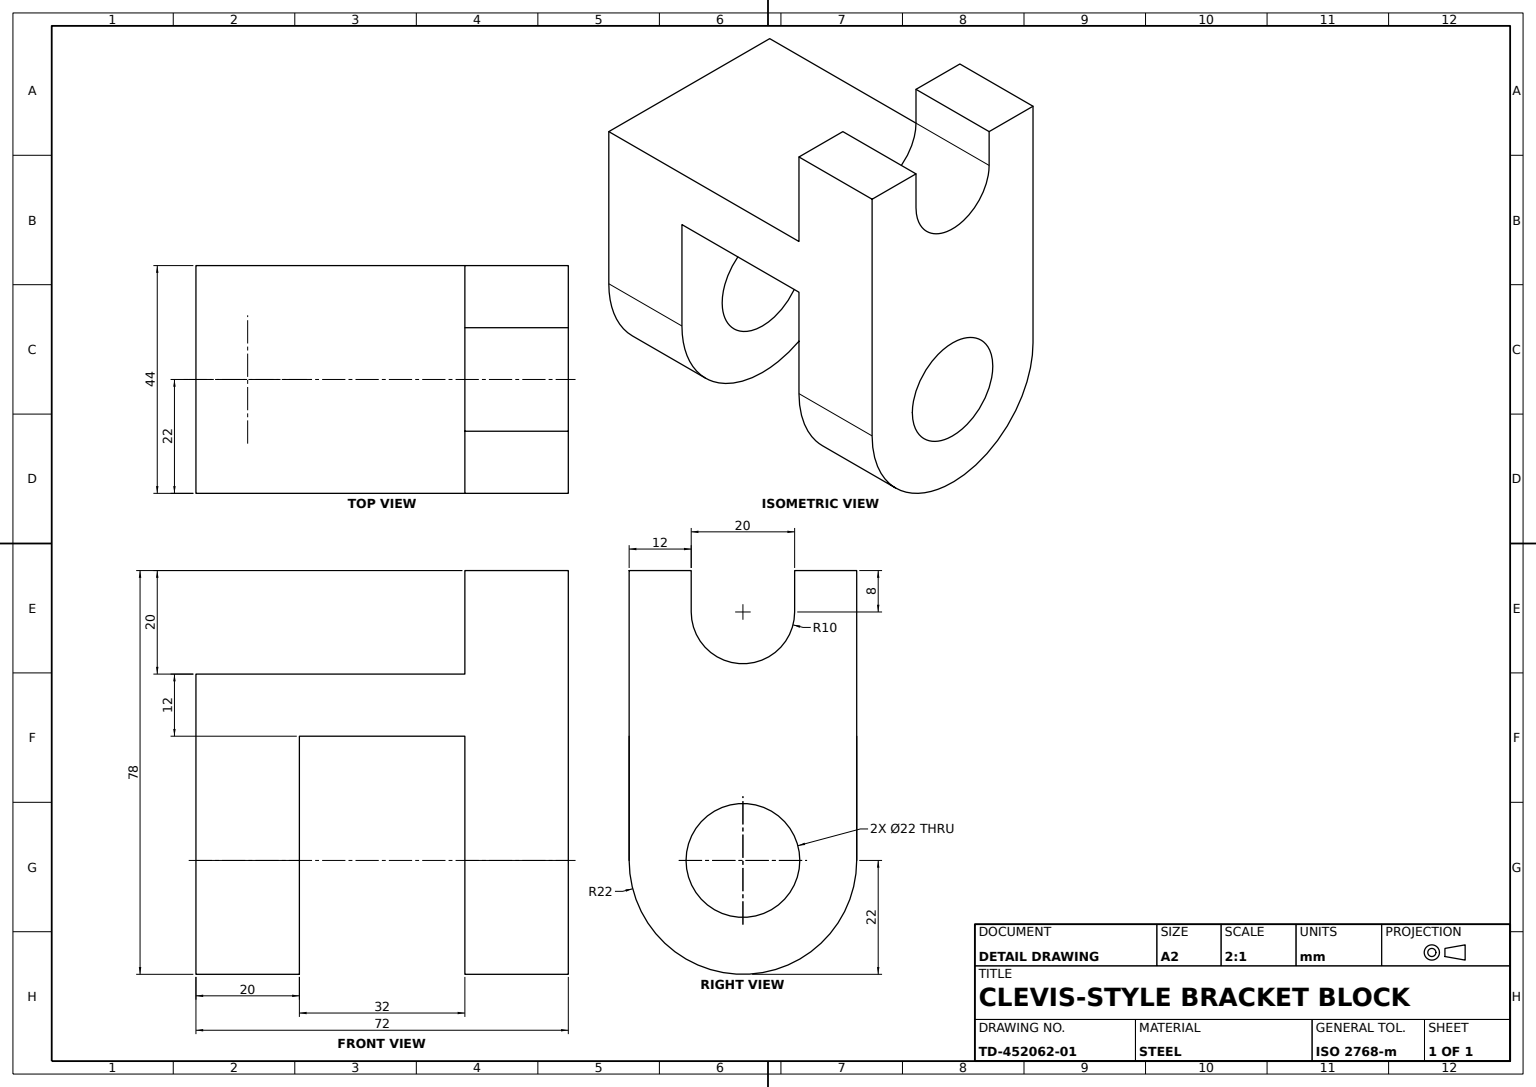
from build123d import *

# Parameters (mm, degrees)
BASE_BLOCK_DEPTH       = 22
LUG_WEB_SKETCH_W       = 20
LUG_WEB_SKETCH_H       = 44
LUG_WEB_DEPTH          = 24
LUG_BOSS_1_SKETCH_R    = 22
LUG_BOSS_1_SKETCH_R_2  = 11
LUG_BOSS_1_R22_DEPTH   = 20
LUG_HOLE_1_SKETCH_R    = 11
LUG_HOLE_1_DEPTH       = 20
LUG_START              = -20
LUG_BOSS_2_SKETCH_R    = 22
LUG_BOSS_2_SKETCH_R_2  = 11
LUG_BOSS_2_R22_DEPTH   = 20
LUG_HOLE_2_SKETCH_R    = 11
LUG_HOLE_2_DEPTH       = 20
CLEVIS_SLOT_DEPTH      = 73.828565824
CLEVIS_SLOT_DEPTH_BACK = 20


with BuildPart() as part:
    # Base Profile Sketch → Base Block (new, symmetric)
    with BuildSketch(Plane.XY):
        Polygon((-36, 0), (36, 0), (36, 32), (16, 32), (16, 12), (-36, 12), align=None)
    extrude(amount=BASE_BLOCK_DEPTH, both=True)

    # Lug Web Sketch → Lug Web (add)
    with BuildSketch(Plane.XZ):
        with Locations((-26, 0)):
            Rectangle(LUG_WEB_SKETCH_W, LUG_WEB_SKETCH_H)
        with Locations((26, 0)):
            Rectangle(LUG_WEB_SKETCH_W, LUG_WEB_SKETCH_H)
    extrude(amount=LUG_WEB_DEPTH)

    # Lug Boss 1 Sketch → Lug Boss 1 R22 (add)
    with BuildSketch(Plane.ZY.offset(36)):
        with Locations((0, -24)):
            Circle(LUG_BOSS_1_SKETCH_R)
        with Locations((0, -24)):
            Circle(LUG_BOSS_1_SKETCH_R_2, mode=Mode.SUBTRACT)
    extrude(amount=-LUG_BOSS_1_R22_DEPTH)

    # Lug Hole 1 Sketch → Lug Hole 1 (cut)
    with BuildSketch(Plane.ZY.offset(36)):
        with Locations(Location((0, -24, 0), (0, 0, 270))):
            Circle(LUG_HOLE_1_SKETCH_R)
    extrude(amount=-LUG_HOLE_1_DEPTH, mode=Mode.SUBTRACT)

    # Lug Boss 2 Sketch → Lug Boss 2 R22 (add)
    with BuildSketch(Plane(origin=(36, 0, 0), x_dir=(0, 0, -1), z_dir=(1, 0, 0)).offset(LUG_START)):
        with Locations((0, -24)):
            Circle(LUG_BOSS_2_SKETCH_R)
        with Locations(Location((0, -24, 0), (0, 0, 270))):
            Circle(LUG_BOSS_2_SKETCH_R_2, mode=Mode.SUBTRACT)
    extrude(amount=LUG_BOSS_2_R22_DEPTH)

    # Lug Hole 2 Sketch → Lug Hole 2 (cut)
    with BuildSketch(Plane(origin=(36, 0, 0), x_dir=(0, 0, -1), z_dir=(1, 0, 0)).offset(LUG_START)):
        with Locations(Location((0, -24, 0), (0, 0, 270))):
            Circle(LUG_HOLE_2_SKETCH_R)
    extrude(amount=LUG_HOLE_2_DEPTH, mode=Mode.SUBTRACT)

    # Clevis Slot Sketch → Clevis Slot (cut, two sides: drawn at the far end of the back side and taken through both)
    with BuildSketch(Plane.ZY.offset(-16).offset(-CLEVIS_SLOT_DEPTH_BACK)):
        with BuildLine():
            Line((-10, 32), (-10, 24))
            ThreePointArc((-10, 24), (0, 14), (10, 24))
            Line((10, 24), (10, 32))
            Line((10, 32), (-10, 32))
        make_face()
    extrude(amount=CLEVIS_SLOT_DEPTH + CLEVIS_SLOT_DEPTH_BACK, mode=Mode.SUBTRACT)


solid = part.part
